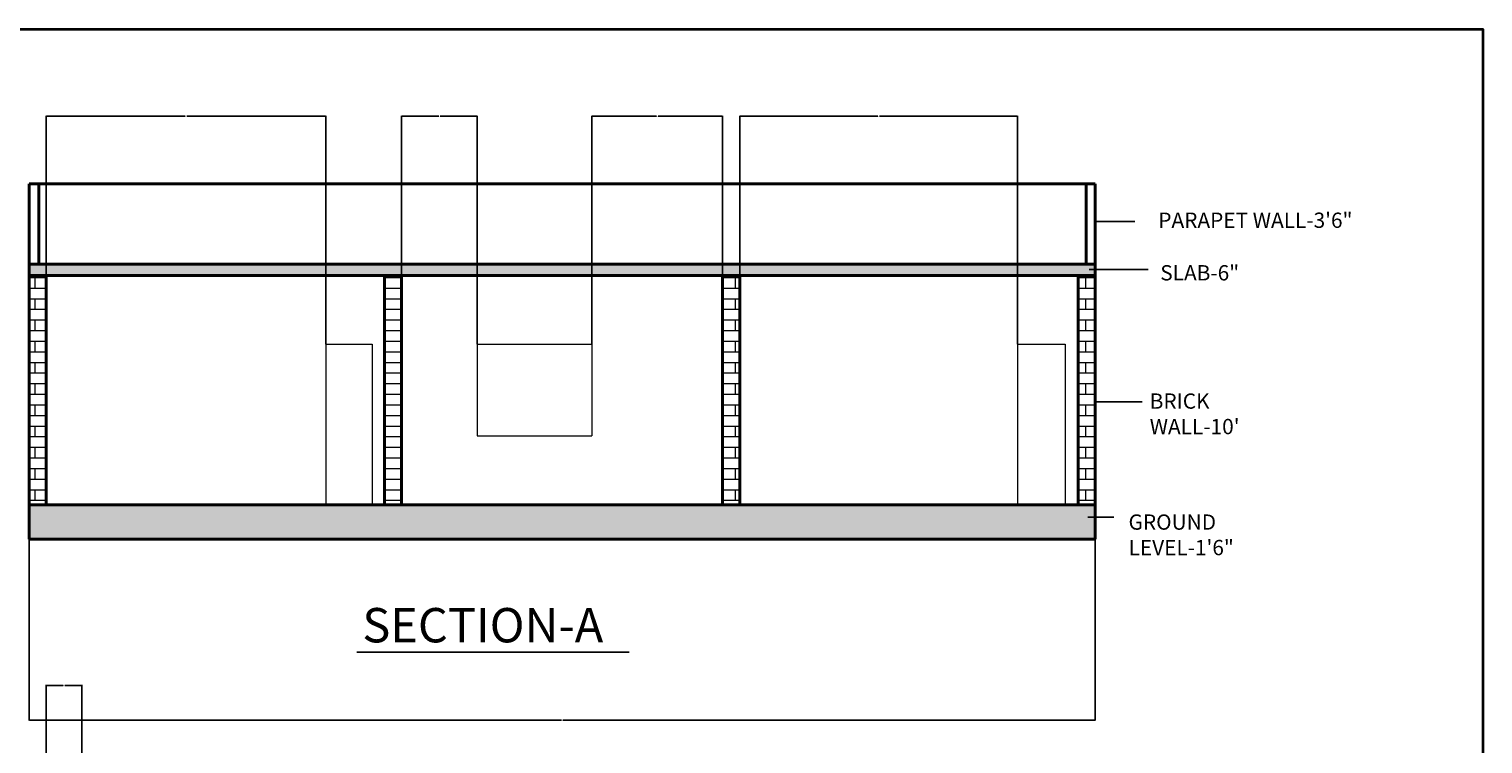
# Model space of a CAD drawing. Units: inches. Extents: x 2215 to 3724, y 1009 to 2124.
# Tile 11 of 11: x 2963 to 3724, y 1750 to 2124. Entities that reach past the tile are written whole.
import ezdxf

# ---------------------------------------------------------------- set-up
doc = ezdxf.new("R2010")
doc.units = ezdxf.units.IN
for name, color, linetype, lineweight in [('A-ANNO-DIMS', 2, 'Continuous', 18), ('A-ANNO-TEXT', 7, 'Continuous', 25), ('A-ANNO-TTLB', 7, 'Continuous', 35), ('A-SECT', 7, 'Continuous', 40), ('A-SECT-BYND', 7, 'Continuous', 18), ('A-SECT-PATT', 8, 'Continuous', 13), ('A-WALL-PATT', 8, 'Continuous', 13)]:
    doc.layers.add(name, color=color, linetype=linetype, lineweight=lineweight)
doc.styles.get("Standard").update_dxf_attribs({"font": 'arial.ttf'})
doc.dimstyles.get("Standard").update_dxf_attribs({"dimtxt": 0.18, "dimasz": 0.18, "dimexe": 0.18, "dimexo": 0.0625, "dimgap": 0.09, "dimtad": 0, "dimtih": 1, "dimtoh": 1, "dimdec": 4, "dimzin": 0, "dimdsep": 46, "dimtxsty": 'Standard', "dimcen": 0.09, "dimadec": 0, "dimazin": 0, "dimtfac": 1, "dimtdec": 4, "dimtofl": 0, "dimtmove": 0, "dimatfit": 3, "dimfxl": 1, "dimtolj": 1, "dimtzin": 0, "dimarcsym": 0})

# ---------------------------------------------------------------- blocks, each defined once
blk = doc.blocks.new('*D117')
at = {"layer": 'A-ANNO-DIMS', "color": 0, "lineweight": -2, "transparency": 16777216}
for p, q in [((2962.74, 1857.17), (2962.74, 1762.29)), ((3520.74, 1857.17), (3520.74, 1762.29)), ((2962.92, 1762.47), (3241.45, 1762.47)), ((3520.56, 1762.47), (3242.03, 1762.47))]:
    blk.add_line(p, q, dxfattribs=at)
at = {"layer": 'A-ANNO-DIMS', "color": 0, "transparency": 16777216}
for points in [[(2962.92, 1762.5), (2962.92, 1762.44), (2962.74, 1762.47)], [(3520.56, 1762.5), (3520.56, 1762.44), (3520.74, 1762.47)]]:
    blk.add_solid(points, dxfattribs=at)
at = {"layer": 'Defpoints', "color": 0, "transparency": 16777216}
for p in [(2962.74, 1857.24), (3520.74, 1857.24), (3520.74, 1762.47)]:
    blk.add_point(p, dxfattribs=at)
at = {"layer": 'A-ANNO-DIMS', "color": 0, "transparency": 16777216, "insert": (3241.74, 1762.47), "char_height": 0.18, "attachment_point": 5}
blk.add_mtext('\\A1;558', dxfattribs=at)
blk = doc.blocks.new('*D119')
at = {"layer": 'A-ANNO-DIMS', "color": 0, "lineweight": -2, "transparency": 16777216}
for p, q in [((2971.74, 1995.3), (2971.74, 2078.92)), ((2971.92, 2078.74), (3044.45, 2078.74)), ((3117.89, 2078.74), (3045.36, 2078.74)), ((3118.07, 1959.3), (3118.07, 2078.92))]:
    blk.add_line(p, q, dxfattribs=at)
at = {"layer": 'A-ANNO-DIMS', "color": 0, "transparency": 16777216}
for points in [[(2971.92, 2078.77), (2971.92, 2078.71), (2971.74, 2078.74)], [(3117.89, 2078.77), (3117.89, 2078.71), (3118.07, 2078.74)]]:
    blk.add_solid(points, dxfattribs=at)
at = {"layer": 'Defpoints', "color": 0, "transparency": 16777216}
for p in [(3118.07, 2078.74), (2971.74, 1995.24), (3118.07, 1959.24)]:
    blk.add_point(p, dxfattribs=at)
at = {"layer": 'A-ANNO-DIMS', "color": 0, "transparency": 16777216, "insert": (3044.91, 2078.74), "char_height": 0.18, "attachment_point": 5}
blk.add_mtext('\\A1;146.33', dxfattribs=at)
blk = doc.blocks.new('*D120')
at = {"layer": 'A-ANNO-DIMS', "color": 0, "lineweight": -2, "transparency": 16777216}
for p, q in [((3157.74, 1995.3), (3157.74, 2078.92)), ((3157.92, 2078.74), (3177.17, 2078.74)), ((3197.17, 2078.74), (3177.92, 2078.74)), ((3197.35, 1959.3), (3197.35, 2078.92))]:
    blk.add_line(p, q, dxfattribs=at)
at = {"layer": 'A-ANNO-DIMS', "color": 0, "transparency": 16777216}
for points in [[(3157.92, 2078.77), (3157.92, 2078.71), (3157.74, 2078.74)], [(3197.17, 2078.77), (3197.17, 2078.71), (3197.35, 2078.74)]]:
    blk.add_solid(points, dxfattribs=at)
at = {"layer": 'Defpoints', "color": 0, "transparency": 16777216}
for p in [(3197.35, 2078.74), (3157.74, 1995.24), (3197.35, 1959.24)]:
    blk.add_point(p, dxfattribs=at)
at = {"layer": 'A-ANNO-DIMS', "color": 0, "transparency": 16777216, "insert": (3177.55, 2078.74), "char_height": 0.18, "attachment_point": 5}
blk.add_mtext('\\A1;39.61', dxfattribs=at)
blk = doc.blocks.new('*D121')
at = {"layer": 'A-ANNO-DIMS', "color": 0, "lineweight": -2, "transparency": 16777216}
for p, q in [((3257.35, 1959.3), (3257.35, 2078.92)), ((3257.53, 2078.74), (3291.15, 2078.74)), ((3325.56, 2078.74), (3291.94, 2078.74)), ((3325.74, 1995.3), (3325.74, 2078.92))]:
    blk.add_line(p, q, dxfattribs=at)
at = {"layer": 'A-ANNO-DIMS', "color": 0, "transparency": 16777216}
for points in [[(3257.53, 2078.77), (3257.53, 2078.71), (3257.35, 2078.74)], [(3325.56, 2078.77), (3325.56, 2078.71), (3325.74, 2078.74)]]:
    blk.add_solid(points, dxfattribs=at)
at = {"layer": 'Defpoints', "color": 0, "transparency": 16777216}
for p in [(3325.74, 2078.74), (3325.74, 1995.24), (3257.35, 1959.24)]:
    blk.add_point(p, dxfattribs=at)
at = {"layer": 'A-ANNO-DIMS', "color": 0, "transparency": 16777216, "insert": (3291.55, 2078.74), "char_height": 0.18, "attachment_point": 5}
blk.add_mtext('\\A1;68.39', dxfattribs=at)
blk = doc.blocks.new('*D122')
at = {"layer": 'A-ANNO-DIMS', "color": 0, "lineweight": -2, "transparency": 16777216}
for p, q in [((3334.74, 1995.3), (3334.74, 2078.92)), ((3334.92, 2078.74), (3406.98, 2078.74)), ((3479.94, 2078.74), (3407.89, 2078.74)), ((3480.12, 1959.3), (3480.12, 2078.92))]:
    blk.add_line(p, q, dxfattribs=at)
at = {"layer": 'A-ANNO-DIMS', "color": 0, "transparency": 16777216}
for points in [[(3334.92, 2078.77), (3334.92, 2078.71), (3334.74, 2078.74)], [(3479.94, 2078.77), (3479.94, 2078.71), (3480.12, 2078.74)]]:
    blk.add_solid(points, dxfattribs=at)
at = {"layer": 'Defpoints', "color": 0, "transparency": 16777216}
for p in [(3480.12, 2078.74), (3334.74, 1995.24), (3480.12, 1959.24)]:
    blk.add_point(p, dxfattribs=at)
at = {"layer": 'A-ANNO-DIMS', "color": 0, "transparency": 16777216, "insert": (3407.43, 2078.74), "char_height": 0.18, "attachment_point": 5}
blk.add_mtext('\\A1;145.37', dxfattribs=at)
blk = doc.blocks.new('*D127')
at = {"layer": 'A-ANNO-DIMS', "color": 0, "lineweight": -2, "transparency": 16777216}
for p, q in [((2971.74, 1440.06), (2971.74, 1780.83)), ((2971.92, 1780.65), (2980.62, 1780.65)), ((2990.24, 1780.65), (2981.53, 1780.65)), ((2990.42, 1440.06), (2990.42, 1780.83))]:
    blk.add_line(p, q, dxfattribs=at)
at = {"layer": 'A-ANNO-DIMS', "color": 0, "transparency": 16777216}
for points in [[(2971.92, 1780.68), (2971.92, 1780.62), (2971.74, 1780.65)], [(2990.24, 1780.68), (2990.24, 1780.62), (2990.42, 1780.65)]]:
    blk.add_solid(points, dxfattribs=at)
at = {"layer": 'Defpoints', "color": 0, "transparency": 16777216}
for p in [(2990.42, 1780.65), (2971.74, 1440), (2990.42, 1440)]:
    blk.add_point(p, dxfattribs=at)
at = {"layer": 'A-ANNO-DIMS', "color": 0, "transparency": 16777216, "insert": (2981.08, 1780.65), "char_height": 0.18, "attachment_point": 5}
blk.add_mtext('\\A1;18.673', dxfattribs=at)

msp = doc.modelspace()

# ---------------------------------------------------------------- hatches: boundary and pattern name
at = {"layer": 'A-SECT-PATT'}
h = msp.add_hatch(dxfattribs=at)
h.set_pattern_fill('AR-CONC', color=256, scale=0.048, style=0)
h.paths.add_polyline_path([(2962.7432, 1995.2374), (3520.7432, 1995.2374), (3520.7432, 2001.2374), (2962.7432, 2001.2374)])
h = msp.add_hatch(dxfattribs=at)
h.set_pattern_fill('AR-CONC', color=256, scale=0.12, style=0)
h.paths.add_polyline_path([(2962.7432, 1857.2374), (3520.7432, 1857.2374), (3520.7432, 1875.2374), (2962.7432, 1875.2374)])
at = {"layer": 'A-WALL-PATT'}
h = msp.add_hatch(dxfattribs=at)
h.set_pattern_fill('AR-BRSTD', color=256, scale=0.082, style=0)
h.paths.add_polyline_path([(2962.7432, 1875.2374), (2971.7432, 1875.2374), (2971.7432, 1995.2374), (2962.7432, 1995.2374)])
h = msp.add_hatch(dxfattribs=at)
h.set_pattern_fill('AR-BRSTD', color=256, scale=0.082, style=0)
h.paths.add_polyline_path([(3148.7432, 1875.2374), (3157.7432, 1875.2374), (3157.7432, 1995.2374), (3148.7432, 1995.2374)])
h = msp.add_hatch(dxfattribs=at)
h.set_pattern_fill('AR-BRSTD', color=256, scale=0.082, style=0)
h.paths.add_polyline_path([(3325.7432, 1875.2374), (3334.7432, 1875.2374), (3334.7432, 1995.2374), (3325.7432, 1995.2374)])
h = msp.add_hatch(dxfattribs=at)
h.set_pattern_fill('AR-BRSTD', color=256, scale=0.082, style=0)
h.paths.add_polyline_path([(3511.7432, 1875.2374), (3520.7432, 1875.2374), (3520.7432, 1995.2374), (3511.7432, 1995.2374)])

# ---------------------------------------------------------------- linework, layer by layer
at = {"layer": 'A-ANNO-TEXT'}
for p, q in [((3520.7432, 2023.488), (3541.5589, 2023.488)), ((3517.5869, 1998.4417), (3548.5014, 1998.4417)), ((3520.7432, 1929.063), (3545.3654, 1929.063)), ((3516.8358, 1868.787), (3530.4915, 1868.787)), ((3134.3651, 1797.9722), (3276.8432, 1797.9722))]:
    msp.add_line(p, q, dxfattribs=at)
at = {"layer": 'A-ANNO-TTLB'}
msp.add_lwpolyline([(2215.4438, 2124.2681), (3723.6589, 2124.2681), (3723.6589, 1008.7935), (2215.4438, 1008.7935)], close=True, dxfattribs=at)
at = {"layer": 'A-SECT'}
for p, q in [((2962.7432, 2043.2374), (2962.7432, 1857.2374)), ((2962.7432, 2043.2374), (3520.7432, 2043.2374)), ((2967.8821, 2001.2374), (2967.8821, 2043.2374)), ((3515.9994, 2001.2374), (3515.9994, 2043.2374)), ((3520.7432, 2043.2374), (3520.7432, 1857.2374)), ((2962.7432, 2001.2374), (3520.7432, 2001.2374)), ((2962.7432, 1995.2374), (3520.7432, 1995.2374)), ((2971.7432, 1995.2374), (2971.7432, 1875.2374)), ((3148.7432, 1995.2374), (3148.7432, 1875.2374)), ((3157.7432, 1995.2374), (3157.7432, 1875.2374)), ((3325.7432, 1995.2374), (3325.7432, 1875.2374)), ((3334.7432, 1995.2374), (3334.7432, 1875.2374)), ((3511.7432, 1995.2374), (3511.7432, 1875.2374)), ((2962.7432, 1875.2374), (3520.7432, 1875.2374)), ((2962.7432, 1857.2374), (3520.7432, 1857.2374))]:
    msp.add_line(p, q, dxfattribs=at)
at = {"layer": 'A-SECT-BYND'}
for p, q in [((3118.074, 1959.2374), (3142.3342, 1959.2374)), ((3118.074, 1959.2374), (3118.074, 1875.2374)), ((3142.3342, 1959.2374), (3142.3342, 1875.2374)), ((3197.3513, 1959.2374), (3197.3513, 1911.2374)), ((3197.3513, 1959.2374), (3257.3513, 1959.2374)), ((3257.3513, 1959.2374), (3257.3513, 1911.2374)), ((3480.1173, 1959.2374), (3480.1173, 1875.2374)), ((3480.1173, 1959.2374), (3504.954, 1959.2374)), ((3504.954, 1959.2374), (3504.954, 1875.2374)), ((3197.3513, 1911.2374), (3257.3513, 1911.2374))]:
    msp.add_line(p, q, dxfattribs=at)

# ---------------------------------------------------------------- texts
at = {"layer": 'A-ANNO-TEXT', "attachment_point": 1}
for s, width, insert, char_height in [('PARAPET WALL-3\'6"', 181.832473, (3553.7569, 2028.1835), 8), ('SLAB-6"', 50.174932, (3554.7957, 2000.656), 8), ("BRICK WALL-10'", 58.396698, (3549.2592, 1933.4864), 8), ('GROUND LEVEL-1\'6"', 74.996777, (3538.179, 1870.1329), 8), ('SECTION-A', 316.61553, (3137.1584, 1821.1345), 18)]:
    msp.add_mtext_dynamic_manual_height_columns(s, width=width, gutter_width=12.5, heights=[0], dxfattribs=dict(at, insert=insert, char_height=char_height))

# ---------------------------------------------------------------- dimensions: what is measured, and where the dimension line sits
at = {"layer": 'A-ANNO-DIMS'}
for base, p1, p2, override, picture, middle in [((3118.074, 2078.7374), (2971.7432, 1995.2374), (3118.074, 1959.2374), {"dimdec": 2, "dimlfac": 1, "dimrnd": 0, "dimzin": 0, "dimdsep": 46, "dimlunit": 2}, '*D119', (3044.9086, 2078.7374)), ((3197.3513, 2078.7374), (3157.7432, 1995.2374), (3197.3513, 1959.2374), {"dimdec": 2, "dimlfac": 1, "dimrnd": 0, "dimzin": 0, "dimdsep": 46, "dimlunit": 2}, '*D120', (3177.5473, 2078.7374)), ((3325.7432, 2078.7374), (3257.3513, 1959.2374), (3325.7432, 1995.2374), {"dimdec": 2, "dimlfac": 1, "dimrnd": 0, "dimzin": 0, "dimdsep": 46, "dimlunit": 2}, '*D121', (3291.5473, 2078.7374)), ((3480.1173, 2078.7374), (3334.7432, 1995.2374), (3480.1173, 1959.2374), {"dimdec": 2, "dimlfac": 1, "dimrnd": 0, "dimzin": 0, "dimdsep": 46, "dimlunit": 2}, '*D122', (3407.4302, 2078.7374)), ((3520.7432, 1762.4722), (2962.7432, 1857.2374), (3520.7432, 1857.2374), {"dimdec": 0, "dimlfac": 1, "dimrnd": 0, "dimzin": 0, "dimdsep": 46, "dimlunit": 2}, '*D117', (3241.7432, 1762.4722)), ((2990.4162, 1780.6469), (2971.7432, 1439.9969), (2990.4162, 1439.9969), {"dimdec": 3, "dimlfac": 1, "dimrnd": 0, "dimzin": 0, "dimdsep": 46, "dimlunit": 2}, '*D127', (2981.0797, 1780.6469))]:
    dim = msp.add_linear_dim(base=base, p1=p1, p2=p2, dimstyle='Standard', override=override, dxfattribs=at)
    dim.commit()
    dim.dimension.update_dxf_attribs({"geometry": picture, "text_midpoint": middle})

doc.saveas('drawing.dxf')
